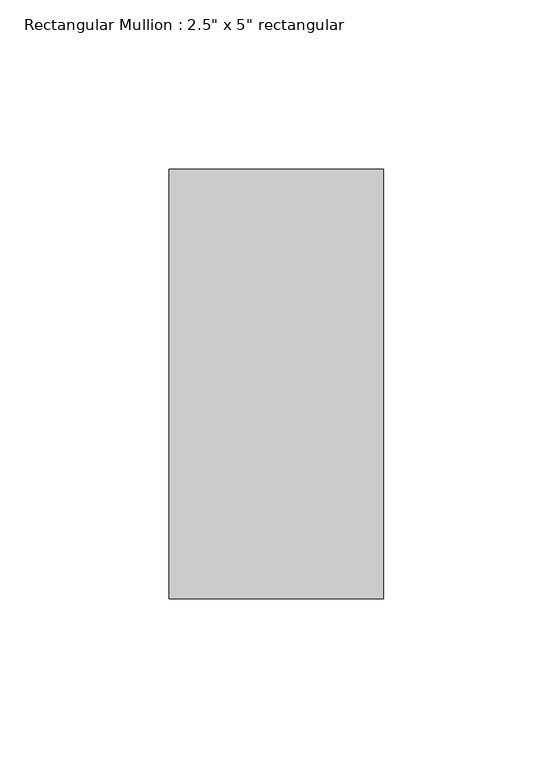
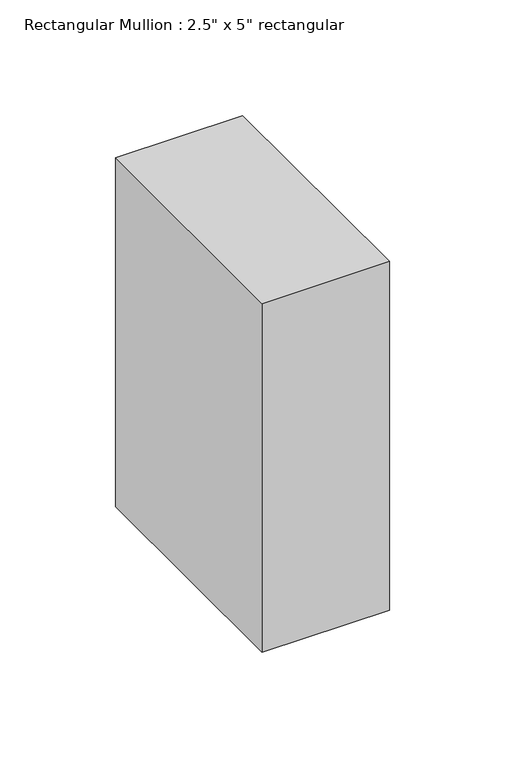
"""IFC4 building model written with IfcOpenShell, lengths in millimetres: member geometry."""

from ifc_helpers import new_model, si_unit, frame, origin, place, context, project, spatial, polyline, outline, extrude, source, transform, mapped, element, save


def member_9890e23f(model_context):
    return source(origin(), model_context, "Body", "SweptSolid", [
        extrude(outline(polyline([(0.0, 63.5), (0.0, -63.5), (-63.5, -63.5), (-63.5, 63.5), (0.0, 63.5)])), frame((0.0, 0.0, -184.15), z_axis=(0.0, 0.0, 1.0), x_axis=(1.0, 0.0, 0.0)), (0.0, 0.0, 1.0), 184.15),
    ])


if __name__ == "__main__":
    model = new_model("IFC4")
    model_context = context("Model", 3, world=origin())
    ifc_project = project(units=[si_unit("LENGTHUNIT", "METRE", prefix="MILLI")], contexts=[model_context])
    site = spatial("IfcSite", under=ifc_project)
    building = spatial("IfcBuilding", under=site)
    placement = place(None, origin())
    member_shape = member_9890e23f(model_context)
    element("IfcMember", 1, ObjectType="Rectangular Mullion : 2.5\" x 5\" rectangular", at=placement, inside=building, context=model_context, shape_type="MappedRepresentation", body=[
        mapped(member_shape, transform((0.0, 0.0, 0.0), x_axis=(1.0, 0.0, 0.0), y_axis=(0.0, 1.0, 0.0), z_axis=(0.0, 0.0, 1.0))),
    ])
    save(model, "model.ifc")

# Revit data of these elements
# Type "Rectangular Mullion : 2.5\" x 5\" rectangular"
#   built-in parameter 1007304 = 0.416667 (stored number, unit not read)
#   built-in parameter 1007301 = 0.104167 (stored number, unit not read)
#   built-in parameter 1007300 = 0.104167 (stored number, unit not read)
# Element 1 (IfcMember, "Rectangular Mullion : 2.5\" x 5\" rectangular")
#   Materials on its faces: "Aluminum"
# Materials
#   "Aluminum": class "Metal", colour RGB 247 247 247, transparency 0, Description = "Aluminum 6061", Cost = 0
